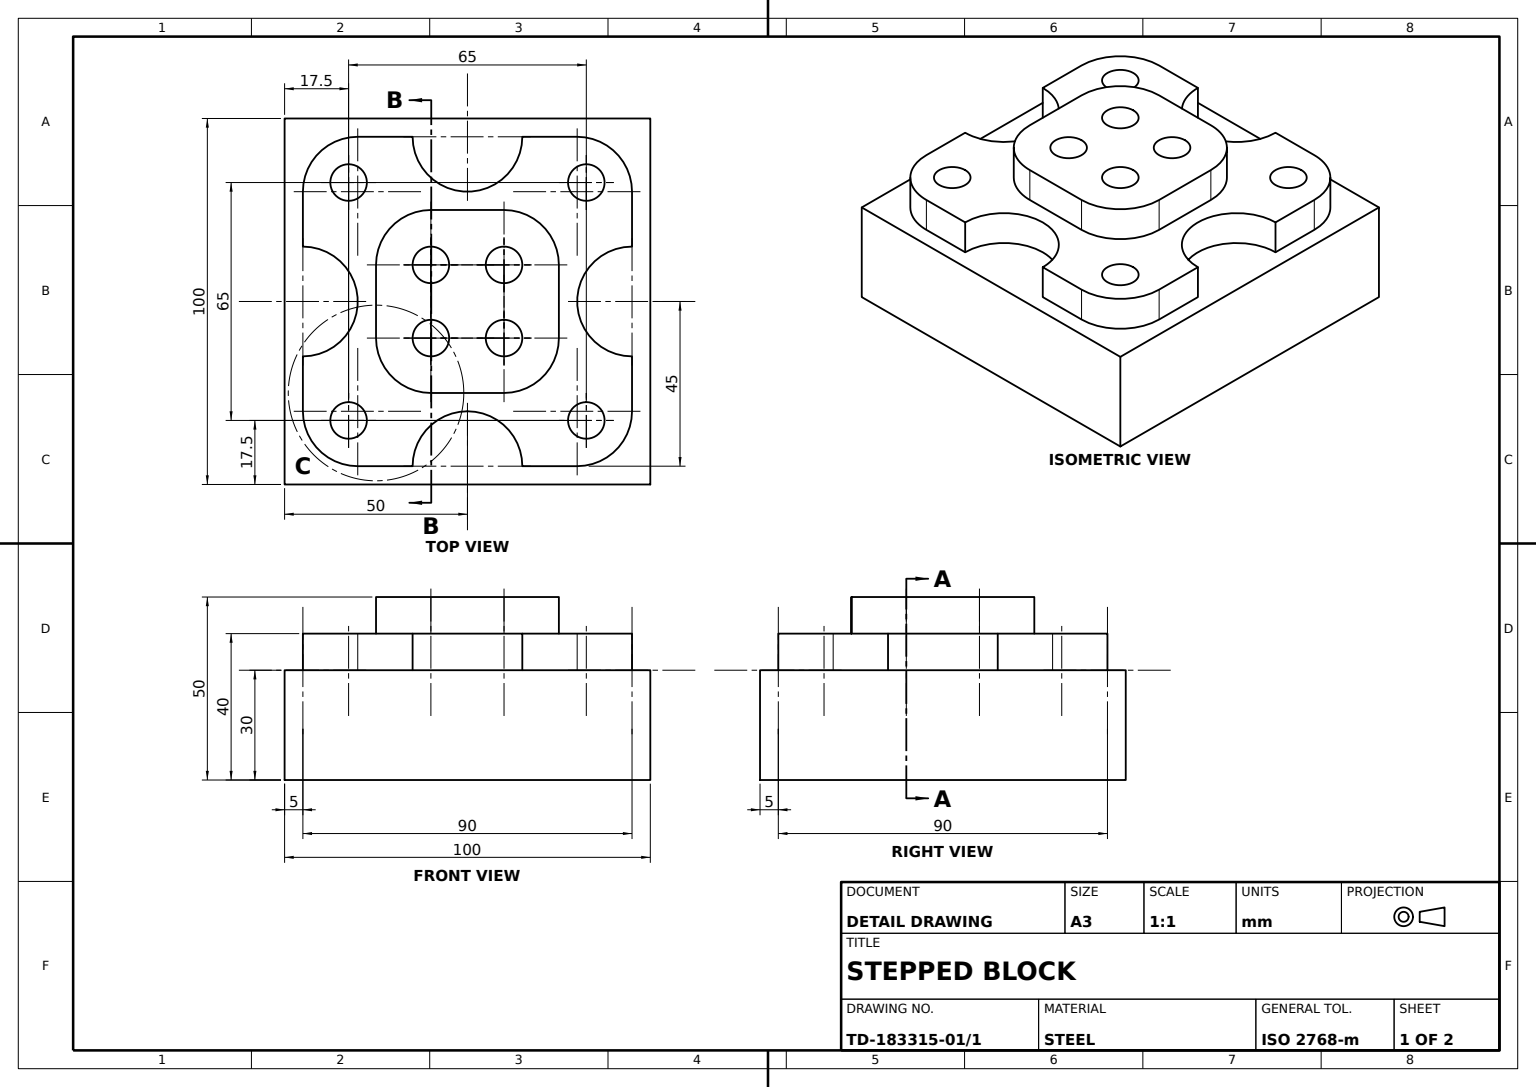
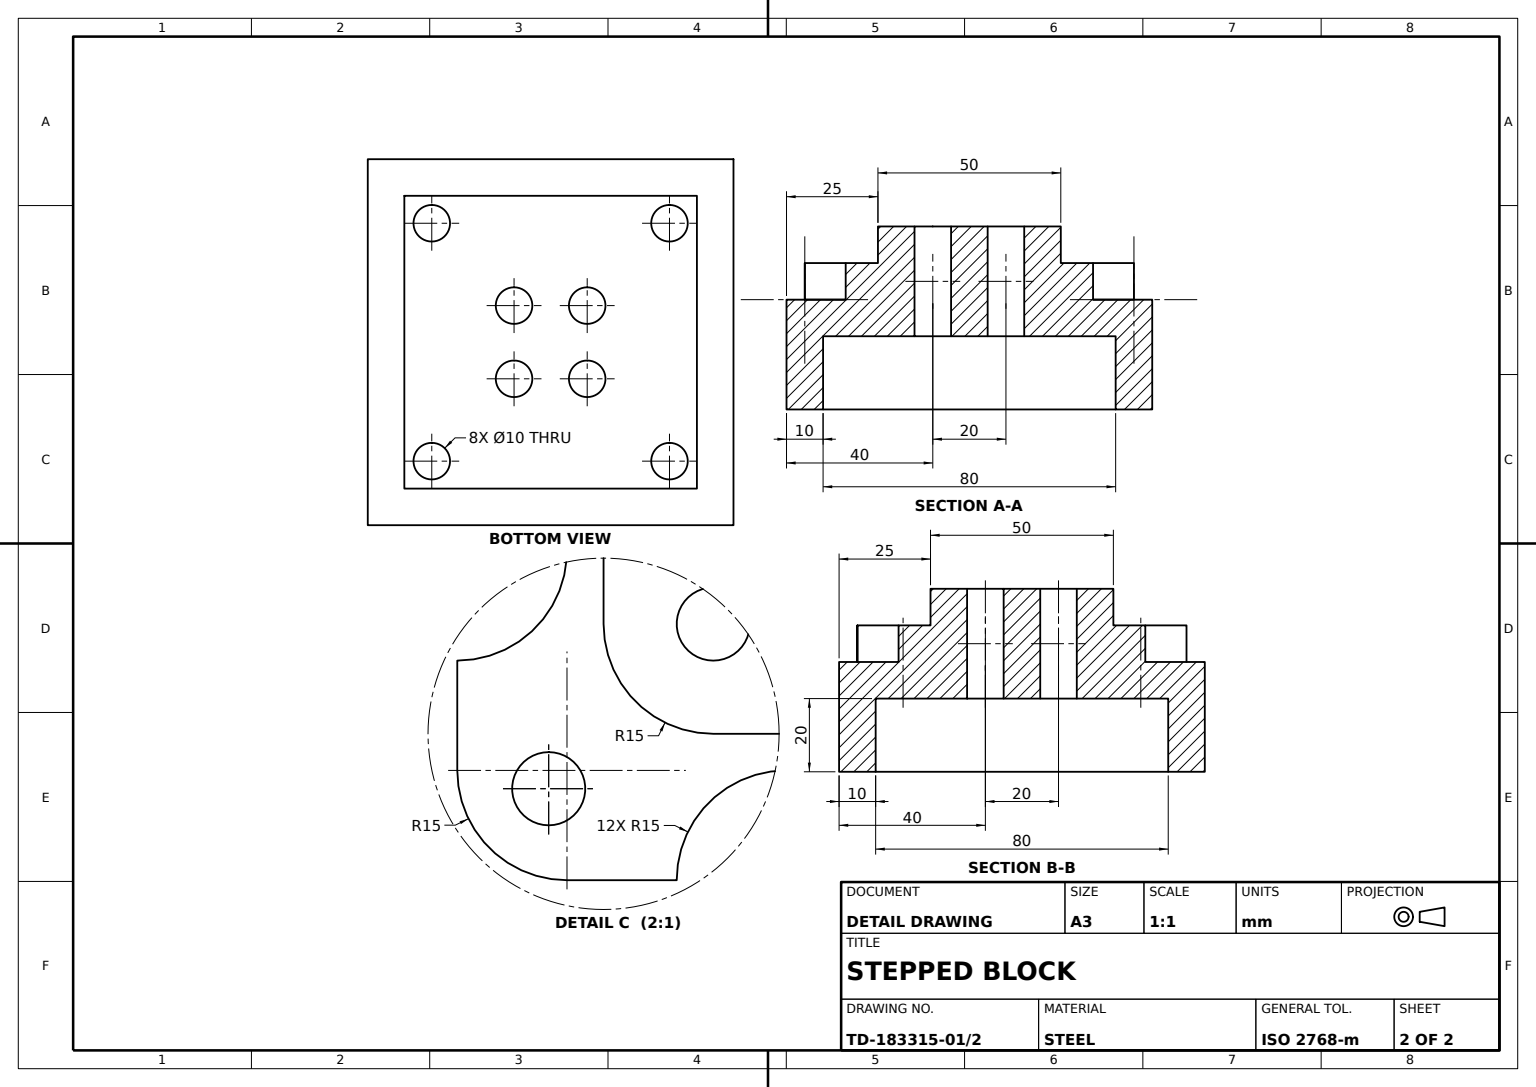
SolidWorks part; units mm, degrees
material "Plain Carbon Steel"
ref_plane "Front Plane" through (0, 0, 0) normal (0, 0, 1) x (1, 0, 0)
ref_plane "Top Plane" through (0, 0, 0) normal (0, 1, 0) x (1, 0, 0)
ref_plane "Right Plane" through (0, 0, 0) normal (1, 0, 0) x (0, 0, -1)
sketch "Base Square Sketch" plane through (0, 0, 0) normal (0, 1, 0) x (1, 0, 0)
  line L1 (-50, -50) -> (50, -50)
  line L2 (-50, -50) -> (-50, 50)
  line L3 (-50, 50) -> (50, 50)
  line L4 (50, -50) -> (50, 50)
  line L5 (-50, -50) -> (50, 50) construction
  line L6 (-50, 50) -> (50, -50) construction
  point P0 (0, 0)
  dimension "D1" = 100
extrude "Base Block 100x100x30" add sketch "Base Square Sketch" along normal blind 30
shell "Base Shell 10mm" thickness 10
sketch "Cross Plate Sketch" plane through (0, 30, 0) normal (0, 1, 0) x (1, 0, 0)
  line L0 (15, 45) -> (30, 45)
  line L1 (-30, -45) -> (-15, -45)
  line L2 (-45, -30) -> (-45, -15)
  line L3 (-30, 45) -> (-15, 45)
  line L4 (45, -30) -> (45, -15)
  line L5 (-45, -45) -> (45, 45) construction
  line L6 (-45, 45) -> (45, -45) construction
  line L7 (-45, 15) -> (-45, 30)
  line L8 (45, 15) -> (45, 30)
  line L9 (15, -45) -> (30, -45)
  line L15 (-32.5, -32.5) -> (32.5, 32.5) construction
  line L16 (-32.5, 32.5) -> (32.5, -32.5) construction
  arc A0 (-30, -45) -> (-45, -30) centre (-30, -30) cw
  arc A1 (30, -45) -> (45, -30) centre (30, -30) ccw
  arc A2 (30, 45) -> (45, 30) centre (30, 30) cw
  arc A3 (-45, 30) -> (-30, 45) centre (-30, 30) cw
  arc A4 (-15, 45) -> (15, 45) centre (0, 45) ccw
  arc A5 (45, 15) -> (45, -15) centre (45, 0) ccw
  arc A6 (15, -45) -> (-15, -45) centre (0, -45) ccw
  arc A7 (-45, -15) -> (-45, 15) centre (-45, 0) ccw
  circle A8 centre (-32.5, 32.5) radius 5
  circle A9 centre (32.5, 32.5) radius 5
  circle A10 centre (-32.5, -32.5) radius 5
  circle A11 centre (32.5, -32.5) radius 5
  point P0 (0, 0)
  point P19 (0, 0)
  dimension "D2" = 15
  dimension "D3" = 30
  dimension "D5" = 45
  dimension "D7" = 10
  dimension "D8" = 10
  dimension "D9" = 10
  dimension "D10" = 10
  dimension "D1" = 90
  dimension "D4" = 15
  dimension "D11" = 65
  dimension "D12" = 65
  dimension "D13" = 65
  dimension "D14" = 65
  dimension "D15" = 32.5
  dimension "D6" = 4
extrude "Cross Plate 10mm" add sketch "Cross Plate Sketch" along normal blind 10
sketch "Plate Holes Sketch" plane through (0, 40, 0) normal (0, 1, 0) x (1, 0, 0)
  circle A0 centre (-32.5, 32.5) radius 5
  circle A1 centre (32.5, 32.5) radius 5
  circle A2 centre (32.5, -32.5) radius 5
  circle A3 centre (-32.5, -32.5) radius 5
  dimension "D1" = 10
  dimension "D2" = 10
  dimension "D3" = 10
  dimension "D4" = 10
extrude "Plate Arm Holes 4x" cut sketch "Plate Holes Sketch" against normal through all
sketch "Centre Boss Sketch" plane through (0, 40, 0) normal (0, 1, 0) x (1, 0, 0)
  line L0 (-25, 10) -> (-25, -10)
  line L5 (45, -30) -> (45, -15) construction
  line L6 (-30, -45) -> (-15, -45) construction
  line L7 (-10, 25) -> (10, 25)
  line L8 (25, 10) -> (25, -10)
  line L9 (-10, -25) -> (10, -25)
  circle A0 centre (-10, 10) radius 5
  circle A1 centre (10, 10) radius 5
  circle A2 centre (10, -10) radius 5
  circle A3 centre (-10, -10) radius 5
  arc A6 (-25, -10) -> (-10, -25) centre (-10, -10) ccw
  arc A8 (-10, 25) -> (-25, 10) centre (-10, 10) ccw
  arc A10 (25, 10) -> (10, 25) centre (10, 10) ccw
  arc A11 (10, -25) -> (25, -10) centre (10, -10) ccw
  point P0 (0, 0)
  dimension "D3" = 10
  dimension "D4" = 10
  dimension "D5" = 10
  dimension "D6" = 10
  dimension "D7" = 15
  dimension "D1" = 20
  dimension "D2" = 20
  dimension "D8" = 20
  dimension "D9" = 20
extrude "Centre Boss 10mm" add sketch "Centre Boss Sketch" along normal blind 10
sketch "Centre Holes Sketch" plane through (0, 50, 0) normal (0, 1, 0) x (1, 0, 0)
  circle A0 centre (-10, 10) radius 5
  circle A1 centre (10, 10) radius 5
  circle A2 centre (10, -10) radius 5
  circle A3 centre (-10, -10) radius 5
  dimension "D1" = 10
  dimension "D2" = 10
  dimension "D3" = 10
  dimension "D4" = 10
  dimension "D5" = 10
  dimension "D6" = 10
extrude "Centre Boss Holes 4x" cut sketch "Centre Holes Sketch" against normal through all
